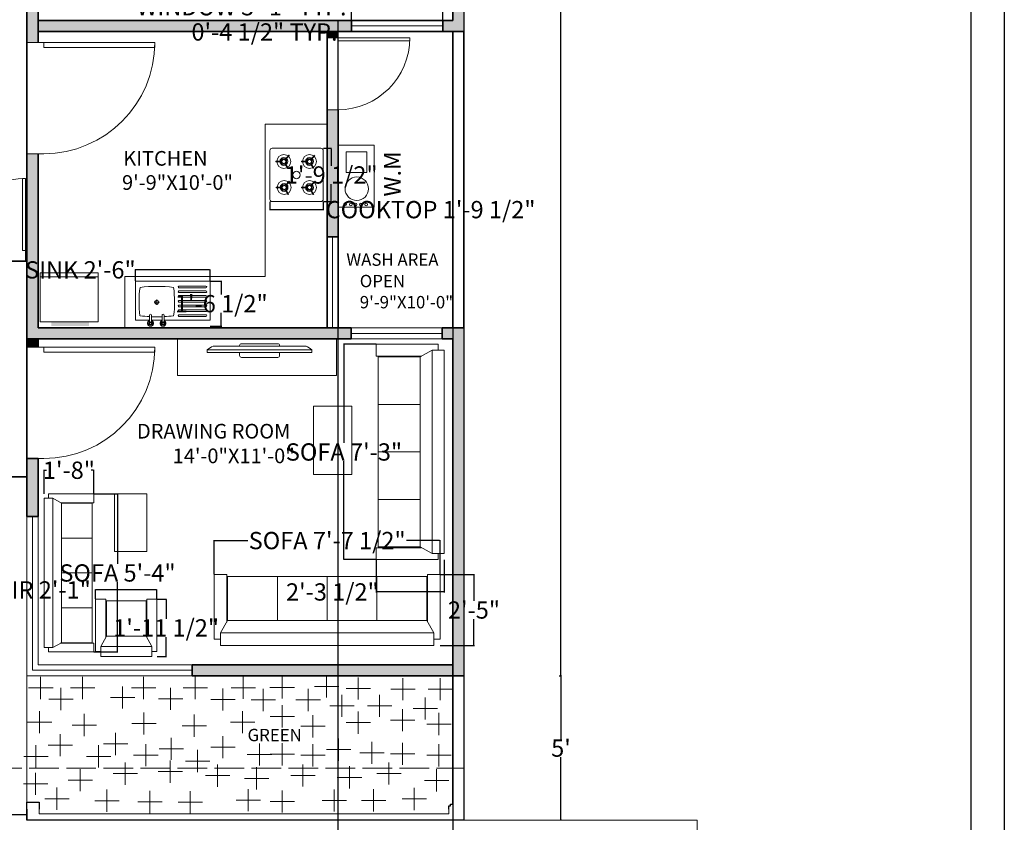
# Model space of a CAD drawing. Units: inches. Extents: x 0 to 4258, y 0 to 3769.
# Tile 18 of 30: x 3859 to 4258, y 2936 to 3261. Entities that reach past the tile are written whole.
import ezdxf

# ---------------------------------------------------------------- set-up
doc = ezdxf.new("R2010")
doc.units = ezdxf.units.IN
doc.header["$MEASUREMENT"] = 0
doc.linetypes.add('ACAD_ISO02W100', pattern=[15, 12, -3])
doc.layers.get('0').update_dxf_attribs({"color": 16})
for name, color, linetype, lineweight in [('A-ANNO-DIMS', 250, 'Continuous', 18), ('A-ANNO-TEXT', 250, 'Continuous', 18), ('A-ANNO-TTLB', 250, 'Continuous', 25), ('A-AREA-IDEN', 250, 'Continuous', 18), ('A-CASE', 150, 'Continuous', 18), ('A-EQPM', 8, 'Continuous', 18), ('A-FLOR-FIXT', 250, 'Continuous', 18), ('A-FLOR-OVHD', 150, 'ACAD_ISO02W100', 13), ('A-FLOR-STRS', 150, 'Continuous', 25), ('A-WALL-PATT', 16, 'Continuous', 13), ('C-PROP', 150, 'Continuous', 25), ('C-ROAD', 250, 'Continuous', 18), ('doors', 250, 'Continuous', 18), ('furniture', 13, 'Continuous', 18), ('L-PLNT-GRND', 102, 'Continuous', 13), ('walls', 251, 'Continuous', 35), ('windows', 121, 'Continuous', 18)]:
    doc.layers.add(name, color=color, linetype=linetype, lineweight=lineweight)
doc.styles.get("Standard").update_dxf_attribs({"font": 'arial.ttf'})
doc.dimstyles.get("Standard").update_dxf_attribs({"dimtxt": 7, "dimasz": 0.18, "dimexe": 0.18, "dimexo": 0.0625, "dimgap": 0.09, "dimtad": 0, "dimtih": 1, "dimtoh": 1, "dimzin": 0, "dimdsep": 46, "dimlunit": 3, "dimtxsty": 'Standard', "dimcen": 0.09, "dimadec": 0, "dimazin": 0, "dimtfac": 1, "dimtofl": 0, "dimtmove": 0, "dimatfit": 3, "dimfxl": 1, "dimtolj": 1, "dimtzin": 0, "dimarcsym": 0})

# ---------------------------------------------------------------- blocks, each defined once
blk = doc.blocks.new('FABRIC SOFA 4S')
at = {"layer": 'furniture'}
for p, q in [((3, 54), (34, 54)), ((3, 51), (3, 54)), ((34, 48), (34, 54)), ((0, -51), (0, 51)), ((6, 51), (0, 51)), ((6, -51), (6, 51)), ((12, 47.63), (6, 51)), ((11.14, 48), (34, 48)), ((33, 23.81), (12, 23.81)), ((33, 0), (12, 0)), ((33, -23.81), (12, -23.81)), ((6, -51), (0, -51)), ((3, -54), (3, -51)), ((6, -51), (12, -47.63)), ((11.54, -48), (34, -48)), ((34, -48), (34, -54)), ((3, -54), (34, -54))]:
    blk.add_line(p, q, dxfattribs=at)
blk.add_lwpolyline([(12, -47.63), (12, 47.63), (33, 47.63), (33, -47.63)], close=True, dxfattribs=at)
blk = doc.blocks.new('A$C799204C7')
for p, q in [((0, 34.2), (17.99, 34.2)), ((0, 0), (0, 34.2)), ((2.32, 20.01), (2.32, 32.27)), ((3.13, 20.01), (3.13, 32.27)), ((4.48, 20.01), (4.48, 32.27)), ((5.29, 20.01), (5.29, 32.27)), ((6.64, 20.01), (6.64, 32.27)), ((7.45, 20.01), (7.45, 32.27)), ((8.85, 20.01), (8.85, 32.27)), ((9.66, 20.01), (9.66, 32.27)), ((11.01, 20.01), (11.01, 32.27)), ((11.82, 20.01), (11.82, 32.27)), ((13.22, 20.01), (13.22, 32.27)), ((14.03, 20.01), (14.03, 32.27)), ((15.42, 20.01), (15.42, 32.27)), ((16.24, 20.01), (16.24, 32.27)), ((17.99, 13.08), (17.99, 34.2)), ((8.52, 9.77), (10.9, 9.77)), ((9.73, 11), (9.73, 8.54)), ((18.59, 13.08), (15.71, 13.08)), ((15.71, 12.17), (18.59, 12.17)), ((17.99, 7.36), (17.99, 12.17)), ((18.59, 7.36), (15.71, 7.36)), ((15.71, 6.45), (18.59, 6.45)), ((17.99, 0), (17.99, 6.45)), ((0, 0), (17.99, 0))]:
    blk.add_line(p, q)
for centre, radius in [((9.7, 9.77), 0.916), ((19.38, 12.62), 0.684), ((19.38, 12.62), 0.456), ((19.38, 6.91), 0.684), ((19.38, 6.91), 0.456)]:
    blk.add_circle(centre, radius)
for centre, radius, start, end in [((2.72, 32.27), 0.407, 0, 180), ((4.88, 32.27), 0.407, 0, 180), ((7.05, 32.27), 0.407, 0, 180), ((9.25, 32.27), 0.407, 0, 180), ((11.42, 32.27), 0.407, 0, 180), ((13.62, 32.27), 0.407, 0, 180), ((15.83, 32.27), 0.407, 0, 180), ((2.72, 20.01), 0.407, 180, 0), ((4.88, 20.01), 0.407, 180, 0), ((7.05, 20.01), 0.407, 180, 0), ((9.25, 20.01), 0.407, 180, 0), ((11.42, 20.01), 0.407, 180, 0), ((13.62, 20.01), 0.407, 180, 0), ((15.83, 20.01), 0.407, 180, 0), ((67.33, 9.77), 64.88, 173.1952, 186.8048), ((9.53, -30.19), 48.1, 82.3437, 97.8966), ((-48.51, 9.77), 64.88, 2.9208, 6.8048), ((19.38, 12.62), 1.37, 199.6514, 160.3603), ((15.71, 12.62), 0.456, 90, 270), ((-48.51, 9.77), 64.88, 357.8723, 2.115), ((19.38, 12.62), 0.911, 210.3431, 149.7554), ((15.71, 6.91), 0.456, 90, 270), ((-48.51, 9.77), 64.88, 353.1952, 357.0665), ((19.38, 6.91), 1.37, 199.6514, 160.3603), ((19.38, 6.91), 0.911, 210.3431, 149.7554), ((9.53, 49.73), 48.1, 262.1034, 277.6563)]:
    blk.add_arc(centre, radius, start, end)
blk = doc.blocks.new('sink')
at = {"layer": 'furniture'}
for p, q in [((8718164203.894819, -1433730582.369047), (8718164201.504578, -1433730582.369047)), ((8718164202.684322, -1433730581.131674), (8718164202.684322, -1433730583.598095)), ((8718164196.150837, -1433730592.638258), (8718164196.150837, -1433730604.938997)), ((8718164196.967728, -1433730592.638258), (8718164196.967728, -1433730604.938997)), ((8718164198.365185, -1433730592.638258), (8718164198.365185, -1433730604.938997)), ((8718164199.182076, -1433730592.638258), (8718164199.182076, -1433730604.938997)), ((8718164200.579533, -1433730592.638258), (8718164200.579533, -1433730604.938997)), ((8718164201.396423, -1433730592.638258), (8718164201.396423, -1433730604.938997)), ((8718164202.748692, -1433730592.638258), (8718164202.748692, -1433730604.938997)), ((8718164203.565582, -1433730592.638258), (8718164203.565582, -1433730604.938997)), ((8718164204.963041, -1433730592.638258), (8718164204.963041, -1433730604.938997)), ((8718164205.779934, -1433730592.638258), (8718164205.779934, -1433730604.938997)), ((8718164207.1322, -1433730592.638258), (8718164207.1322, -1433730604.938997)), ((8718164207.949093, -1433730592.638258), (8718164207.949093, -1433730604.938997)), ((8718164209.301359, -1433730592.638258), (8718164209.301359, -1433730604.938997)), ((8718164210.118252, -1433730592.638258), (8718164210.118252, -1433730604.938997))]:
    blk.add_line(p, q, dxfattribs=at)
for centre, radius in [((8718164192.998869, -1433730579.495552), 0.685789), ((8718164192.998869, -1433730579.495552), 0.457192), ((8718164192.998869, -1433730585.228166), 0.68579), ((8718164192.998869, -1433730585.228166), 0.68579), ((8718164192.998869, -1433730585.228166), 0.457192), ((8718164202.715019, -1433730582.369047), 0.919003)]:
    blk.add_circle(centre, radius, dxfattribs=at)
for centre, radius, start, end in [((8718164196.559284, -1433730592.638258), 0.41045, 354.3355999, 185.6644001), ((8718164198.77363, -1433730592.638258), 0.41045, 354.3355999, 185.6644001), ((8718164200.98798, -1433730592.638258), 0.41045, 354.3355999, 185.6644001), ((8718164203.157139, -1433730592.638258), 0.41045, 354.3355999, 185.6644001), ((8718164205.371487, -1433730592.638258), 0.41045, 354.3355999, 185.6644001), ((8718164207.540646, -1433730592.640262), 0.41045, 354.3355999, 185.6644001), ((8718164209.709805, -1433730592.640262), 0.41045, 354.3355999, 185.6644001), ((8718164196.559284, -1433730604.938997), 0.408445, 180, 0), ((8718164198.77363, -1433730604.938997), 0.408445, 180, 0), ((8718164200.98798, -1433730604.938997), 0.408445, 180, 0), ((8718164203.157139, -1433730604.938997), 0.408445, 180, 0), ((8718164205.371487, -1433730604.938997), 0.408445, 180, 0), ((8718164207.540646, -1433730604.938997), 0.408445, 180, 0), ((8718164209.709805, -1433730604.938997), 0.408445, 180, 0)]:
    blk.add_arc(centre, radius, start, end, dxfattribs=at)
at = {"layer": 'furniture', "xscale": 1.0032, "yscale": 1.0032, "zscale": 1.0032, "rotation": 180}
blk.add_blockref('A$C799204C7', (8718164212.441259, -1433730572.566334), dxfattribs=at)
blk = doc.blocks.new('washbasin')
at = {"layer": 'furniture'}
blk.add_blockref('sink', (-8718164214.119328, 1433730589.721069), dxfattribs=at)
blk = doc.blocks.new('4bstove')
at = {"layer": 'furniture'}
for p, q in [((1452.73, 1446.21), (1452.73, 1448.61)), ((1452.98, 1446.22), (1452.98, 1448.61)), ((1464.44, 1446.34), (1464.44, 1448.73)), ((1464.69, 1446.34), (1464.69, 1448.73)), ((1451.74, 1444.45), (1449.67, 1443.25)), ((1451.87, 1444.23), (1449.79, 1443.04)), ((1453.75, 1444.08), (1455.58, 1442.54)), ((1453.91, 1444.27), (1455.74, 1442.73)), ((1463.45, 1444.58), (1461.38, 1443.38)), ((1463.57, 1444.36), (1461.5, 1443.17)), ((1465.46, 1444.21), (1467.29, 1442.67)), ((1465.62, 1444.4), (1467.45, 1442.86)), ((1452.69, 1434.81), (1452.69, 1437.2)), ((1452.94, 1434.81), (1452.94, 1437.2)), ((1464.44, 1434.81), (1464.44, 1437.2)), ((1464.69, 1434.81), (1464.69, 1437.2)), ((1451.7, 1433.04), (1449.63, 1431.85)), ((1451.82, 1432.83), (1449.75, 1431.63)), ((1453.71, 1432.67), (1455.54, 1431.13)), ((1453.87, 1432.86), (1455.7, 1431.33)), ((1463.45, 1433.04), (1461.38, 1431.85)), ((1463.57, 1432.83), (1461.5, 1431.63)), ((1465.46, 1432.67), (1467.29, 1431.13)), ((1465.62, 1432.86), (1467.45, 1431.33))]:
    blk.add_line(p, q, dxfattribs=at)
for points in [[(1447.5, 1427.38), (1469.5, 1427.38, 0.414214), (1470.5, 1428.38), (1470.5, 1450.38, 0.414214), (1469.5, 1451.38), (1447.5, 1451.38, 0.414214), (1446.5, 1450.38), (1446.5, 1428.38, 0.414214)], [(1453.75, 1444.97, 1), (1452, 1444.97, 1)], [(1465.46, 1445.1, 1), (1463.71, 1445.1, 1)], [(1453.71, 1433.56, 1), (1451.96, 1433.56, 1)], [(1465.46, 1433.56, 1), (1463.71, 1433.56, 1)]]:
    blk.add_lwpolyline(points, format="xyb", close=True, dxfattribs=at)
for points in [[(1454.12, 1444.97, 1), (1451.62, 1444.97, 1), (1454.12, 1444.97, 1)], [(1465.83, 1445.1, 1), (1463.33, 1445.1, 1), (1465.83, 1445.1, 1)], [(1454.08, 1433.56, 1), (1451.58, 1433.56, 1), (1454.08, 1433.56, 1)], [(1465.83, 1433.56, 1), (1463.33, 1433.56, 1), (1465.83, 1433.56, 1)]]:
    blk.add_lwpolyline(points, format="xyb", dxfattribs=at)
for centre, radius in [((1452.87, 1444.97), 3.14), ((1452.87, 1444.97), 1.75), ((1464.58, 1445.1), 3.14), ((1464.58, 1445.1), 1.75), ((1458.5, 1439.38), 1.67), ((1452.83, 1433.56), 3.14), ((1464.58, 1433.56), 3.14), ((1452.83, 1433.56), 1.75), ((1464.58, 1433.56), 1.75)]:
    blk.add_circle(centre, radius, dxfattribs=at)
for centre, start, end in [((1452.87, 1444.97), 88.2645, 92.2039), ((1464.58, 1445.1), 88.2645, 92.2039), ((1452.87, 1444.97), 208.188, 212.1274), ((1452.87, 1444.97), 318.1018, 322.0412), ((1464.58, 1445.1), 208.188, 212.1274), ((1464.58, 1445.1), 318.1018, 322.0412), ((1452.83, 1433.56), 88.2645, 92.2039), ((1464.58, 1433.56), 88.2645, 92.2039)]:
    blk.add_arc(centre, 3.64, start, end, dxfattribs=at)
blk = doc.blocks.new('stove')
at = {"layer": 'furniture', "xscale": 0.9, "yscale": 0.9, "zscale": 0.9, "rotation": 89.99999999999999}
blk.add_blockref('4bstove', (1295.44, -1312.65), dxfattribs=at)
blk = doc.blocks.new('FABRIC SOFA 1S')
at = {"layer": 'furniture'}
for p, q in [((3, 18.12), (34, 18.12)), ((3, 15.12), (3, 18.12)), ((34, 12.12), (34, 18.12)), ((0, -15.12), (0, 15.12)), ((6, 15.12), (0, 15.12)), ((6, -15.12), (6, 15.12)), ((12, 11.75), (6, 15.12)), ((11.33, 12.12), (34, 12.12)), ((6, -15.12), (0, -15.12)), ((3, -18.12), (3, -15.12)), ((6, -15.12), (12, -11.75)), ((11.33, -12.12), (34, -12.12)), ((34, -12.12), (34, -18.12)), ((3, -18.12), (34, -18.12))]:
    blk.add_line(p, q, dxfattribs=at)
blk.add_lwpolyline([(12, -11.75), (12, 11.75), (33, 11.75), (33, -11.75)], close=True, dxfattribs=at)
blk = doc.blocks.new('PLASMA-LARGE')
at = {"layer": 'furniture'}
for p, q in [((-7.26, 0), (7.26, 0)), ((-21, -2.5), (21, -2.5)), ((-21, -2.5), (-21, -3.5)), ((-21, -3.5), (21, -3.5)), ((-18.61, -1), (18.61, -1)), ((-8, -1), (-8, -0.74)), ((-8, -3.5), (-8, -4.76)), ((8, -1), (8, -0.74)), ((8, -3.5), (8, -4.76)), ((21, -2.5), (21, -3.5)), ((-7.26, -5.5), (7.26, -5.5))]:
    blk.add_line(p, q, dxfattribs=at)
for centre, radius, start, end in [((-7.26, -0.74), 0.744, 90, 180), ((7.26, -0.74), 0.744, 0, 90), ((-13.97, -11.05), 11.07, 114.7602, 129.4175), ((13.97, -11.05), 11.07, 50.5825, 65.2398), ((-7.26, -4.76), 0.744, 180, 270), ((7.26, -4.76), 0.744, 270, 0)]:
    blk.add_arc(centre, radius, start, end, dxfattribs=at)
blk = doc.blocks.new('*U23')
for p, q in [((0, 0), (0, -6)), ((40, 0), (40, -6))]:
    blk.add_line(p, q)
blk.add_lwpolyline([(0, 0), (0, 40), (1.75, 40), (1.75, 0)], close=True)
blk.add_arc((0, 0), 40, 0, 90)
blk = doc.blocks.new('*D26')
at = {"layer": 'A-ANNO-DIMS', "color": 0, "lineweight": -2, "transparency": 16777216}
for p, q in [((4077.41, 3656.79), (4078.27, 3656.79)), ((4078.09, 3656.61), (4078.09, 3329.69)), ((4078.09, 2995.47), (4078.09, 3322.39)), ((4077.41, 2995.29), (4078.27, 2995.29))]:
    blk.add_line(p, q, dxfattribs=at)
at = {"layer": 'A-ANNO-DIMS', "color": 0, "transparency": 16777216}
for points in [[(4078.06, 3656.61), (4078.12, 3656.61), (4078.09, 3656.79)], [(4078.06, 2995.47), (4078.12, 2995.47), (4078.09, 2995.29)]]:
    blk.add_solid(points, dxfattribs=at)
at = {"layer": 'Defpoints', "color": 0, "transparency": 16777216}
for p in [(4077.35, 3656.79), (4077.35, 2995.29), (4078.09, 2995.29)]:
    blk.add_point(p, dxfattribs=at)
at = {"layer": 'A-ANNO-DIMS', "color": 0, "transparency": 16777216, "insert": (4078.09, 3326.04), "char_height": 7, "attachment_point": 5}
blk.add_mtext("\\A1;55'", dxfattribs=at)
blk = doc.blocks.new('*D27')
at = {"layer": 'A-ANNO-DIMS', "color": 0, "lineweight": -2, "transparency": 16777216}
for p, q in [((4078.25, 2995.29), (4077.91, 2995.29)), ((4078.09, 2995.11), (4078.09, 2969.69)), ((4078.09, 2936.97), (4078.09, 2962.39)), ((4078.25, 2936.79), (4077.91, 2936.79))]:
    blk.add_line(p, q, dxfattribs=at)
at = {"layer": 'A-ANNO-DIMS', "color": 0, "transparency": 16777216}
for points in [[(4078.06, 2995.11), (4078.12, 2995.11), (4078.09, 2995.29)], [(4078.06, 2936.97), (4078.12, 2936.97), (4078.09, 2936.79)]]:
    blk.add_solid(points, dxfattribs=at)
at = {"layer": 'Defpoints', "color": 0, "transparency": 16777216}
for p in [(4078.31, 2995.29), (4078.09, 2936.79), (4078.31, 2936.79)]:
    blk.add_point(p, dxfattribs=at)
at = {"layer": 'A-ANNO-DIMS', "color": 0, "transparency": 16777216, "insert": (4078.09, 2966.04), "char_height": 7, "width": 37.9222, "attachment_point": 5}
blk.add_mtext("\\A1;5'", dxfattribs=at)
blk = doc.blocks.new('WINDOW-37IN')
for p, q in [((0, 4.5), (36.9, 4.5)), ((0, 2.25), (36.9, 2.25)), ((0, 0), (36.9, 0))]:
    blk.add_line(p, q)
blk = doc.blocks.new('TV-CONSOLE-CABINET')
for p, q in [((0, 0), (0, 64.44)), ((0, 64.44), (14.9, 64.44)), ((14.9, 0), (0, 0))]:
    blk.add_line(p, q)
blk = doc.blocks.new('LAWN-COVER-MARK')
for p, q in [((4.88, 8.97), (4.88, 0)), ((0, 4.49), (9.88, 4.49))]:
    blk.add_line(p, q)
blk = doc.blocks.new('*D40')
at = {"layer": 'A-ANNO-DIMS', "color": 0, "lineweight": -2, "transparency": 16777216}
for p, q in [((3937.65, 3036.44), (3937.65, 3050.28)), ((3937.83, 3050.1), (3951.19, 3050.1)), ((4028.95, 3050.1), (4015.59, 3050.1)), ((4029.13, 3036.44), (4029.13, 3050.28))]:
    blk.add_line(p, q, dxfattribs=at)
at = {"layer": 'A-ANNO-DIMS', "color": 0, "transparency": 16777216}
for points in [[(3937.83, 3050.13), (3937.83, 3050.07), (3937.65, 3050.1)], [(4028.95, 3050.13), (4028.95, 3050.07), (4029.13, 3050.1)]]:
    blk.add_solid(points, dxfattribs=at)
at = {"layer": 'Defpoints', "color": 0, "transparency": 16777216}
for p in [(3937.65, 3050.1), (3937.65, 3036.38), (4029.13, 3036.38)]:
    blk.add_point(p, dxfattribs=at)
at = {"layer": 'A-ANNO-DIMS', "color": 0, "transparency": 16777216, "insert": (3983.39, 3050.1), "char_height": 7, "attachment_point": 5}
blk.add_mtext('\\A1;SOFA 7\'-7 1/2"', dxfattribs=at)
blk = doc.blocks.new('*D41')
at = {"layer": 'A-ANNO-DIMS', "color": 0, "lineweight": -2, "transparency": 16777216}
for p, q in [((4029.19, 3036.38), (4043.03, 3036.38)), ((4042.85, 3036.2), (4042.85, 3025.65)), ((4042.85, 3007.76), (4042.85, 3018.32)), ((4029.19, 3007.58), (4043.03, 3007.58))]:
    blk.add_line(p, q, dxfattribs=at)
at = {"layer": 'A-ANNO-DIMS', "color": 0, "transparency": 16777216}
for points in [[(4042.82, 3036.2), (4042.88, 3036.2), (4042.85, 3036.38)], [(4042.82, 3007.76), (4042.88, 3007.76), (4042.85, 3007.58)]]:
    blk.add_solid(points, dxfattribs=at)
at = {"layer": 'Defpoints', "color": 0, "transparency": 16777216}
for p in [(4029.13, 3036.38), (4042.85, 3036.38), (4029.13, 3007.58)]:
    blk.add_point(p, dxfattribs=at)
at = {"layer": 'A-ANNO-DIMS', "color": 0, "transparency": 16777216, "insert": (4042.85, 3021.98), "char_height": 7, "attachment_point": 5}
blk.add_mtext('\\A1;2\'-5"', dxfattribs=at)
blk = doc.blocks.new('*D42')
at = {"layer": 'A-ANNO-DIMS', "color": 0, "lineweight": -2, "transparency": 16777216}
for p, q in [((4003.23, 3129.61), (3990.02, 3129.61)), ((3990.2, 3129.43), (3990.2, 3089.71)), ((3990.2, 3042.56), (3990.2, 3082.28)), ((4003.23, 3042.38), (3990.02, 3042.38))]:
    blk.add_line(p, q, dxfattribs=at)
at = {"layer": 'A-ANNO-DIMS', "color": 0, "transparency": 16777216}
for points in [[(3990.17, 3129.43), (3990.23, 3129.43), (3990.2, 3129.61)], [(3990.17, 3042.56), (3990.23, 3042.56), (3990.2, 3042.38)]]:
    blk.add_solid(points, dxfattribs=at)
at = {"layer": 'Defpoints', "color": 0, "transparency": 16777216}
for p in [(3990.2, 3129.61), (4003.29, 3129.61), (4003.29, 3042.38)]:
    blk.add_point(p, dxfattribs=at)
at = {"layer": 'A-ANNO-DIMS', "color": 0, "transparency": 16777216, "insert": (3990.2, 3085.99), "char_height": 7, "attachment_point": 5}
blk.add_mtext('\\A1;SOFA 7\'-3"', dxfattribs=at)
blk = doc.blocks.new('*D43')
at = {"layer": 'A-ANNO-DIMS', "color": 0, "lineweight": -2, "transparency": 16777216}
for p, q in [((4003.29, 3042.32), (4003.29, 3029.11)), ((4030.75, 3042.32), (4030.75, 3029.11)), ((4003.29, 3029.29), (4003.11, 3029.29)), ((4030.57, 3029.29), (4003.47, 3029.29))]:
    blk.add_line(p, q, dxfattribs=at)
at = {"layer": 'A-ANNO-DIMS', "color": 0, "transparency": 16777216}
for points in [[(4003.47, 3029.32), (4003.47, 3029.26), (4003.29, 3029.29)], [(4030.57, 3029.32), (4030.57, 3029.26), (4030.75, 3029.29)]]:
    blk.add_solid(points, dxfattribs=at)
at = {"layer": 'Defpoints', "color": 0, "transparency": 16777216}
for p in [(4003.29, 3042.38), (4030.75, 3042.38), (4003.29, 3029.29)]:
    blk.add_point(p, dxfattribs=at)
at = {"layer": 'A-ANNO-DIMS', "color": 0, "transparency": 16777216, "insert": (3985.5, 3029.29), "char_height": 7, "attachment_point": 5}
blk.add_mtext('\\A1;2\'-3 1/2"', dxfattribs=at)
blk = doc.blocks.new('*D44')
at = {"layer": 'A-ANNO-DIMS', "color": 0, "lineweight": -2, "transparency": 16777216}
for p, q in [((3888.92, 3068.99), (3898.64, 3068.99)), ((3898.46, 3068.81), (3898.46, 3040.69)), ((3898.46, 3005.15), (3898.46, 3033.27)), ((3888.92, 3004.97), (3898.64, 3004.97))]:
    blk.add_line(p, q, dxfattribs=at)
at = {"layer": 'A-ANNO-DIMS', "color": 0, "transparency": 16777216}
for points in [[(3898.43, 3068.81), (3898.49, 3068.81), (3898.46, 3068.99)], [(3898.43, 3005.15), (3898.49, 3005.15), (3898.46, 3004.97)]]:
    blk.add_solid(points, dxfattribs=at)
at = {"layer": 'Defpoints', "color": 0, "transparency": 16777216}
for p in [(3888.85, 3068.99), (3888.85, 3004.97), (3898.46, 3004.97)]:
    blk.add_point(p, dxfattribs=at)
at = {"layer": 'A-ANNO-DIMS', "color": 0, "transparency": 16777216, "insert": (3898.46, 3036.98), "char_height": 7, "attachment_point": 5}
blk.add_mtext('\\A1;SOFA 5\'-4"', dxfattribs=at)
blk = doc.blocks.new('*D45')
at = {"layer": 'A-ANNO-DIMS', "color": 0, "lineweight": -2, "transparency": 16777216}
for p, q in [((3868.7, 3069.05), (3868.7, 3078.77)), ((3868.88, 3078.59), (3869.71, 3078.59)), ((3888.67, 3078.59), (3887.84, 3078.59)), ((3888.85, 3069.05), (3888.85, 3078.77))]:
    blk.add_line(p, q, dxfattribs=at)
at = {"layer": 'A-ANNO-DIMS', "color": 0, "transparency": 16777216}
for points in [[(3868.88, 3078.62), (3868.88, 3078.56), (3868.7, 3078.59)], [(3888.67, 3078.62), (3888.67, 3078.56), (3888.85, 3078.59)]]:
    blk.add_solid(points, dxfattribs=at)
at = {"layer": 'Defpoints', "color": 0, "transparency": 16777216}
for p in [(3888.85, 3078.59), (3868.7, 3068.99), (3888.85, 3068.99)]:
    blk.add_point(p, dxfattribs=at)
at = {"layer": 'A-ANNO-DIMS', "color": 0, "transparency": 16777216, "insert": (3878.78, 3078.59), "char_height": 7, "attachment_point": 5}
blk.add_mtext('\\A1;1\'-8"', dxfattribs=at)
blk = doc.blocks.new('*D52')
at = {"layer": 'A-ANNO-DIMS', "color": 0, "lineweight": -2, "transparency": 16777216}
for p, q in [((3889.6, 3030.12), (3889.42, 3030.12)), ((3889.6, 3026.46), (3889.6, 3030.3)), ((3914.27, 3030.12), (3889.78, 3030.12)), ((3914.45, 3026.46), (3914.45, 3030.3))]:
    blk.add_line(p, q, dxfattribs=at)
at = {"layer": 'A-ANNO-DIMS', "color": 0, "transparency": 16777216}
for points in [[(3889.78, 3030.15), (3889.78, 3030.09), (3889.6, 3030.12)], [(3914.27, 3030.15), (3914.27, 3030.09), (3914.45, 3030.12)]]:
    blk.add_solid(points, dxfattribs=at)
at = {"layer": 'Defpoints', "color": 0, "transparency": 16777216}
for p in [(3889.6, 3030.12), (3889.6, 3026.4), (3914.45, 3026.4)]:
    blk.add_point(p, dxfattribs=at)
at = {"layer": 'A-ANNO-DIMS', "color": 0, "transparency": 16777216, "insert": (3852.38, 3030.12), "char_height": 7, "attachment_point": 5}
blk.add_mtext('\\A1;ARMCHAIR 2\'-1"', dxfattribs=at)
blk = doc.blocks.new('*D53')
at = {"layer": 'A-ANNO-DIMS', "color": 0, "lineweight": -2, "transparency": 16777216}
for p, q in [((3914.51, 3026.4), (3918.35, 3026.4)), ((3918.17, 3026.22), (3918.17, 3018.45)), ((3918.17, 3003.27), (3918.17, 3011.03)), ((3914.51, 3003.09), (3918.35, 3003.09))]:
    blk.add_line(p, q, dxfattribs=at)
at = {"layer": 'A-ANNO-DIMS', "color": 0, "transparency": 16777216}
for points in [[(3918.14, 3026.22), (3918.2, 3026.22), (3918.17, 3026.4)], [(3918.14, 3003.27), (3918.2, 3003.27), (3918.17, 3003.09)]]:
    blk.add_solid(points, dxfattribs=at)
at = {"layer": 'Defpoints', "color": 0, "transparency": 16777216}
for p in [(3914.45, 3026.4), (3918.17, 3026.4), (3914.45, 3003.09)]:
    blk.add_point(p, dxfattribs=at)
at = {"layer": 'A-ANNO-DIMS', "color": 0, "transparency": 16777216, "insert": (3918.17, 3014.74), "char_height": 7, "attachment_point": 5}
blk.add_mtext('\\A1;1\'-11 1/2"', dxfattribs=at)
blk = doc.blocks.new('*D58')
at = {"layer": 'A-ANNO-DIMS', "color": 0, "lineweight": -2, "transparency": 16777216}
for p, q in [((3993.31, 3260.86), (3993.31, 3266.51)), ((4030.21, 3260.86), (4030.21, 3266.51)), ((3993.31, 3266.33), (3993.13, 3266.33)), ((4030.03, 3266.33), (3993.49, 3266.33))]:
    blk.add_line(p, q, dxfattribs=at)
at = {"layer": 'A-ANNO-DIMS', "color": 0, "transparency": 16777216}
for points in [[(3993.49, 3266.36), (3993.49, 3266.3), (3993.31, 3266.33)], [(4030.03, 3266.36), (4030.03, 3266.3), (4030.21, 3266.33)]]:
    blk.add_solid(points, dxfattribs=at)
at = {"layer": 'Defpoints', "color": 0, "transparency": 16777216}
for p in [(3993.31, 3266.33), (3993.31, 3260.79), (4030.21, 3260.79)]:
    blk.add_point(p, dxfattribs=at)
at = {"layer": 'A-ANNO-DIMS', "color": 0, "transparency": 16777216, "insert": (3948.75, 3266.33), "char_height": 7, "attachment_point": 5}
blk.add_mtext('\\A1;WINDOW 3\'-1" TYP.', dxfattribs=at)
blk = doc.blocks.new('*D59')
at = {"layer": 'A-ANNO-DIMS', "color": 0, "lineweight": -2, "transparency": 16777216}
for p, q in [((3993.24, 3260.79), (3987.59, 3260.79)), ((3987.77, 3260.61), (3987.77, 3256.47)), ((3993.24, 3256.29), (3987.59, 3256.29)), ((3987.77, 3256.11), (3987.59, 3256.11)), ((3987.77, 3256.29), (3987.77, 3256.11))]:
    blk.add_line(p, q, dxfattribs=at)
at = {"layer": 'A-ANNO-DIMS', "color": 0, "transparency": 16777216}
for points in [[(3987.74, 3260.61), (3987.8, 3260.61), (3987.77, 3260.79)], [(3987.74, 3256.47), (3987.8, 3256.47), (3987.77, 3256.29)]]:
    blk.add_solid(points, dxfattribs=at)
at = {"layer": 'Defpoints', "color": 0, "transparency": 16777216}
for p in [(3993.31, 3260.79), (3987.77, 3256.29), (3993.31, 3256.29)]:
    blk.add_point(p, dxfattribs=at)
at = {"layer": 'A-ANNO-DIMS', "color": 0, "transparency": 16777216, "insert": (3958.01, 3256.11), "char_height": 7, "attachment_point": 5}
blk.add_mtext('\\A1;0\'-4 1/2" TYP.', dxfattribs=at)
blk = doc.blocks.new('*D68')
at = {"layer": 'A-ANNO-DIMS', "color": 0, "lineweight": -2, "transparency": 16777216}
for p, q in [((3905.75, 3159.75), (3905.57, 3159.75)), ((3905.75, 3155.28), (3905.75, 3159.93)), ((3935.79, 3159.75), (3905.93, 3159.75)), ((3935.97, 3155.28), (3935.97, 3159.93))]:
    blk.add_line(p, q, dxfattribs=at)
at = {"layer": 'A-ANNO-DIMS', "color": 0, "transparency": 16777216}
for points in [[(3905.93, 3159.78), (3905.93, 3159.72), (3905.75, 3159.75)], [(3935.79, 3159.78), (3935.79, 3159.72), (3935.97, 3159.75)]]:
    blk.add_solid(points, dxfattribs=at)
at = {"layer": 'Defpoints', "color": 0, "transparency": 16777216}
for p in [(3905.75, 3159.75), (3905.75, 3155.22), (3935.97, 3155.22)]:
    blk.add_point(p, dxfattribs=at)
at = {"layer": 'A-ANNO-DIMS', "color": 0, "transparency": 16777216, "insert": (3883.43, 3159.75), "char_height": 7, "attachment_point": 5}
blk.add_mtext('\\A1;SINK 2\'-6"', dxfattribs=at)
blk = doc.blocks.new('*D69')
at = {"layer": 'A-ANNO-DIMS', "color": 0, "lineweight": -2, "transparency": 16777216}
for p, q in [((3936.03, 3155.22), (3940.69, 3155.22)), ((3940.51, 3155.04), (3940.51, 3149.76)), ((3940.51, 3137.07), (3940.51, 3142.34)), ((3936.03, 3136.89), (3940.69, 3136.89))]:
    blk.add_line(p, q, dxfattribs=at)
at = {"layer": 'A-ANNO-DIMS', "color": 0, "transparency": 16777216}
for points in [[(3940.48, 3155.04), (3940.54, 3155.04), (3940.51, 3155.22)], [(3940.48, 3137.07), (3940.54, 3137.07), (3940.51, 3136.89)]]:
    blk.add_solid(points, dxfattribs=at)
at = {"layer": 'Defpoints', "color": 0, "transparency": 16777216}
for p in [(3935.97, 3155.22), (3940.51, 3155.22), (3935.97, 3136.89)]:
    blk.add_point(p, dxfattribs=at)
at = {"layer": 'A-ANNO-DIMS', "color": 0, "transparency": 16777216, "insert": (3940.51, 3146.05), "char_height": 7, "attachment_point": 5}
blk.add_mtext('\\A1;1\'-6 1/2"', dxfattribs=at)
blk = doc.blocks.new('*D70')
at = {"layer": 'A-ANNO-DIMS', "color": 0, "lineweight": -2, "transparency": 16777216}
for p, q in [((3960.18, 3187.33), (3960.18, 3183.97)), ((3981.78, 3187.33), (3981.78, 3183.97)), ((3960.36, 3184.15), (3981.6, 3184.15)), ((3981.78, 3184.15), (3981.96, 3184.15))]:
    blk.add_line(p, q, dxfattribs=at)
at = {"layer": 'A-ANNO-DIMS', "color": 0, "transparency": 16777216}
for points in [[(3960.36, 3184.18), (3960.36, 3184.12), (3960.18, 3184.15)], [(3981.6, 3184.18), (3981.6, 3184.12), (3981.78, 3184.15)]]:
    blk.add_solid(points, dxfattribs=at)
at = {"layer": 'Defpoints', "color": 0, "transparency": 16777216}
for p in [(3960.18, 3187.39), (3981.78, 3187.39), (3981.78, 3184.15)]:
    blk.add_point(p, dxfattribs=at)
at = {"layer": 'A-ANNO-DIMS', "color": 0, "transparency": 16777216, "insert": (4025.28, 3184.15), "char_height": 7, "attachment_point": 5}
blk.add_mtext('\\A1;COOKTOP 1\'-9 1/2"', dxfattribs=at)
blk = doc.blocks.new('*D71')
at = {"layer": 'A-ANNO-DIMS', "color": 0, "lineweight": -2, "transparency": 16777216}
for p, q in [((3981.85, 3208.99), (3985.2, 3208.99)), ((3985.02, 3208.81), (3985.02, 3201.9)), ((3985.02, 3187.57), (3985.02, 3194.48)), ((3981.85, 3187.39), (3985.2, 3187.39))]:
    blk.add_line(p, q, dxfattribs=at)
at = {"layer": 'A-ANNO-DIMS', "color": 0, "transparency": 16777216}
for points in [[(3984.99, 3208.81), (3985.05, 3208.81), (3985.02, 3208.99)], [(3984.99, 3187.57), (3985.05, 3187.57), (3985.02, 3187.39)]]:
    blk.add_solid(points, dxfattribs=at)
at = {"layer": 'Defpoints', "color": 0, "transparency": 16777216}
for p in [(3981.78, 3208.99), (3985.02, 3208.99), (3981.78, 3187.39)]:
    blk.add_point(p, dxfattribs=at)
at = {"layer": 'A-ANNO-DIMS', "color": 0, "transparency": 16777216, "insert": (3985.02, 3198.19), "char_height": 7, "attachment_point": 5}
blk.add_mtext('\\A1;1\'-9 1/2"', dxfattribs=at)
blk = doc.blocks.new('*D72')
at = {"layer": 'A-ANNO-DIMS', "color": 0, "lineweight": -2, "transparency": 16777216}
for p, q in [((4034.3, 3256.23), (4034.3, 2818.78)), ((3987.71, 3253.71), (3987.71, 2818.78)), ((3987.89, 2818.96), (3990.74, 2818.96)), ((4034.12, 2818.96), (4031.27, 2818.96))]:
    blk.add_line(p, q, dxfattribs=at)
at = {"layer": 'A-ANNO-DIMS', "color": 0, "transparency": 16777216}
for points in [[(3987.89, 2818.99), (3987.89, 2818.93), (3987.71, 2818.96)], [(4034.12, 2818.99), (4034.12, 2818.93), (4034.3, 2818.96)]]:
    blk.add_solid(points, dxfattribs=at)
at = {"layer": 'Defpoints', "color": 0, "transparency": 16777216}
for p in [(4034.3, 3256.29), (3987.71, 3253.78), (4034.3, 2818.96)]:
    blk.add_point(p, dxfattribs=at)
at = {"layer": 'A-ANNO-DIMS', "color": 0, "transparency": 16777216, "insert": (4011.01, 2818.96), "char_height": 7, "attachment_point": 5}
blk.add_mtext('\\A1;3\'-10 1/2"', dxfattribs=at)

msp = doc.modelspace()

# ---------------------------------------------------------------- hatches: boundary and pattern name
at = {"layer": 'A-EQPM'}
h = msp.add_hatch(color=256, dxfattribs=at)
h.dxf.hatch_style = 1
h.paths.add_polyline_path([(3886.878, 3137.07), (3886.878, 3138.634), (3871.646, 3138.634), (3871.646, 3137.07)])
at = {"layer": 'A-WALL-PATT'}
h = msp.add_hatch(color=256, dxfattribs=at)
h.dxf.hatch_style = 1
h.paths.add_polyline_path([(3866.304, 3343.984), (3861.804, 3343.984), (3861.804, 3251.848), (3866.304, 3251.848)])
h.paths.add_polyline_path([(3881.946, 3330.642), (3866.304, 3330.642), (3866.304, 3326.142), (3881.946, 3326.142)])
h.paths.add_polyline_path([(4038.804, 3656.793), (3933.804, 3656.793), (3933.804, 3638.769), (3938.304, 3638.769), (3938.304, 3652.293), (4034.304, 3652.293), (4034.304, 3260.793), (4030.207, 3260.793), (4030.207, 3256.293), (4038.804, 3256.293)])
h = msp.add_hatch(color=256, dxfattribs=at)
h.dxf.hatch_style = 1
h.paths.add_polyline_path([(3993.305, 3260.793), (3866.304, 3260.793), (3866.304, 3256.293), (3993.305, 3256.293)])
h.paths.add_polyline_path([(4038.804, 3136.293), (4030.04, 3136.293), (4030.04, 3131.793), (4034.304, 3131.793), (4034.304, 2995.293), (4038.804, 2995.293)])
h.paths.add_polyline_path([(4034.304, 2999.793), (3928.723, 2999.793), (3928.723, 2995.293), (4034.304, 2995.293)])
h.paths.add_polyline_path([(4014.899, 3187.712), (4014.899, 3210.714), (4004.662, 3210.714), (4004.662, 3187.712)], flags=9)
h = msp.add_hatch(color=256, dxfattribs=at)
h.dxf.hatch_style = 1
h.paths.add_polyline_path([(3987.712, 3256.293), (3983.335, 3256.293), (3983.335, 3253.777), (3987.712, 3253.777)])
h = msp.add_hatch(color=256, dxfattribs=at)
h.dxf.hatch_style = 1
h.paths.add_polyline_path([(3866.304, 3206.808), (3861.804, 3206.808), (3861.804, 3163.293), (3861.804, 3131.793), (3993.138, 3131.793), (3993.138, 3136.293), (3866.304, 3136.293)])
h.paths.add_polyline_path([(3866.304, 3083.341), (3861.804, 3083.341), (3861.804, 3059.818), (3866.304, 3059.818)])
edge = h.paths.add_edge_path()
edge.add_line((3987.712, 3224.597), (3983.335, 3224.597))
edge.add_line((3983.335, 3224.597), (3983.335, 3173.195))
edge.add_line((3983.335, 3173.195), (3987.835, 3173.195))
edge.add_line((3987.835, 3173.195), (3987.835, 3224.597))
edge.add_arc((3987.712, 3253.777), 29.18, 270, 270.24143, ccw=False)
h = msp.add_hatch(color=256, dxfattribs=at)
h.dxf.hatch_style = 1
h.paths.add_polyline_path([(3866.304, 3131.793), (3861.804, 3131.793), (3861.804, 3128.38), (3866.304, 3128.38)])

# ---------------------------------------------------------------- linework, layer by layer
at = {"layer": 'A-ANNO-TTLB'}
for p, q in [((4257.673, 3768.679), (4257.673, 2749.714)), ((4244.279, 2762.335), (4244.279, 3758.41))]:
    msp.add_line(p, q, dxfattribs=at)
at = {"layer": 'A-CASE'}
for p, q in [((3958.264, 3157.012), (3958.264, 3218.827)), ((3958.264, 3218.827), (3983.335, 3218.827)), ((3901.437, 3136.293), (3901.437, 3157.012)), ((3901.437, 3157.012), (3958.264, 3157.012))]:
    msp.add_line(p, q, dxfattribs=at)
at = {"layer": 'A-EQPM'}
for p, q in [((4002.436, 3210.2), (3987.835, 3210.2)), ((3991.119, 3199.188), (3991.119, 3207.524)), ((3991.119, 3207.524), (3999.462, 3207.524)), ((3999.462, 3207.524), (3999.462, 3199.188)), ((4002.436, 3185.144), (4002.436, 3210.2)), ((3999.462, 3199.188), (3991.119, 3199.188)), ((4002.436, 3185.144), (3987.835, 3185.144)), ((3987.835, 3179.127), (3987.835, 3179.127)), ((3867.157, 3158.559), (3890.621, 3158.559)), ((3867.157, 3138.634), (3867.157, 3158.559)), ((3867.157, 3156.965), (3890.621, 3156.965)), ((3890.621, 3158.559), (3890.621, 3138.634)), ((3890.621, 3138.634), (3867.157, 3138.634))]:
    msp.add_line(p, q, dxfattribs=at)
for centre, radius in [((3995.369, 3192.615), 4.752), ((3990.673, 3186.375), 0.542), ((3992.981, 3186.228), 0.542), ((3994.882, 3186.228), 0.542), ((3997.082, 3186.228), 0.542), ((3999.174, 3186.228), 0.542)]:
    msp.add_circle(centre, radius, dxfattribs=at)
at = {"layer": 'A-FLOR-OVHD'}
msp.add_line((3832.744, 2957.868), (4038.804, 2957.868), dxfattribs=at)
at = {"layer": 'A-FLOR-STRS'}
for p, q in [((3861.804, 3075.983), (3828.116, 3075.983)), ((3837.232, 3075.983), (3861.804, 3075.983))]:
    msp.add_line(p, q, dxfattribs=at)
at = {"layer": 'C-PROP'}
for p, q in [((4038.804, 3656.793), (4038.804, 2936.793)), ((4038.804, 2995.293), (4038.804, 2936.793)), ((3861.804, 2944.198), (3866.677, 2944.198)), ((3861.804, 2936.793), (3861.804, 2944.198)), ((3866.677, 2944.198), (3866.677, 2941.293)), ((4034.304, 2943.337), (4034.304, 2944.195)), ((3861.804, 2941.293), (3861.804, 2936.793)), ((4032.616, 2941.293), (4032.616, 2942.716)), ((4032.616, 2942.716), (4033.315, 2942.716)), ((4033.315, 2942.716), (4033.315, 2943.337)), ((4033.315, 2943.337), (4034.304, 2943.337)), ((3771.092, 2939.211), (3861.804, 2939.211)), ((4038.804, 2936.793), (3861.804, 2936.793)), ((4038.804, 2936.793), (3861.804, 2936.793))]:
    msp.add_line(p, q, dxfattribs=at)
at = {"layer": 'C-ROAD'}
for p, q in [((4133.199, 2936.793), (4038.804, 2936.793)), ((4133.199, 2860.957), (4133.199, 2936.793))]:
    msp.add_line(p, q, dxfattribs=at)
at = {"layer": 'furniture'}
for p, q in [((3977.905, 3104.568), (3977.905, 3076.875)), ((3993.43, 3104.568), (3977.905, 3104.568)), ((3993.43, 3076.875), (3993.43, 3104.568)), ((3977.905, 3076.875), (3993.43, 3076.875)), ((3897.304, 3069.01), (3897.304, 3045.642)), ((3910.405, 3069.01), (3897.304, 3069.01)), ((3910.405, 3045.642), (3910.405, 3069.01)), ((3897.304, 3045.642), (3910.405, 3045.642))]:
    msp.add_line(p, q, dxfattribs=at)
at = {"layer": 'L-PLNT-GRND'}
for p, q in [((3861.804, 2995.293), (3861.804, 2941.293)), ((4034.304, 2943.337), (4034.304, 2995.293)), ((3861.804, 2944.198), (3866.677, 2944.198)), ((3866.677, 2944.198), (3866.677, 2939.47)), ((3866.677, 2939.47), (4032.616, 2939.47)), ((4032.616, 2939.47), (4032.616, 2942.716)), ((4032.616, 2942.716), (4033.315, 2942.716)), ((4033.315, 2942.716), (4033.315, 2943.337)), ((4033.315, 2943.337), (4034.304, 2943.337))]:
    msp.add_line(p, q, dxfattribs=at)
at = {"layer": 'walls'}
for p, q in [((4034.304, 3652.293), (4034.304, 3260.793)), ((3861.804, 3598.293), (3861.804, 3163.293)), ((3866.304, 3343.984), (3866.304, 3251.848)), ((3866.304, 3260.793), (4034.304, 3260.793)), ((3993.305, 3260.793), (3993.305, 3256.293)), ((4030.207, 3256.293), (4030.207, 3260.793)), ((3866.304, 3256.293), (4038.804, 3256.293)), ((3983.335, 3256.293), (3983.335, 3136.293)), ((3987.712, 3253.777), (3987.712, 3256.293)), ((4034.304, 3136.293), (4034.304, 3256.293)), ((4034.304, 3256.293), (4034.304, 3136.293)), ((4038.804, 3136.293), (4038.804, 3256.173)), ((3987.835, 3224.597), (3987.835, 3136.293)), ((3866.304, 3206.808), (3866.304, 3136.293)), ((3983.335, 3173.195), (3987.835, 3173.195)), ((3678.804, 3163.293), (3861.804, 3163.293)), ((3861.804, 3163.293), (3861.804, 3059.818)), ((3866.304, 3136.293), (3993.138, 3136.293)), ((3993.138, 3136.293), (3993.138, 3131.793)), ((4030.04, 3136.293), (4030.04, 3131.793)), ((4030.04, 3136.293), (4038.804, 3136.293)), ((3861.804, 3131.793), (3993.138, 3131.793)), ((3866.304, 3131.793), (3866.304, 3128.38)), ((4030.04, 3131.793), (4034.304, 3131.793)), ((4034.304, 3131.793), (4034.304, 2944.195)), ((3866.304, 3083.341), (3861.804, 3083.341)), ((3866.304, 3083.341), (3866.304, 3059.818)), ((3861.804, 3059.818), (3866.304, 3059.818)), ((3928.723, 2999.793), (4034.304, 2999.793)), ((3928.723, 2999.793), (3928.723, 2995.293)), ((3928.723, 2995.293), (4038.804, 2995.293))]:
    msp.add_line(p, q, dxfattribs=at)
at = {"layer": 'windows'}
for p, q in [((3861.804, 3059.818), (3861.804, 2995.293)), ((3864.054, 3059.818), (3864.054, 2997.543)), ((3866.304, 3059.818), (3866.304, 2999.793)), ((3866.304, 2999.793), (3928.723, 2999.793)), ((3861.804, 2995.293), (3928.723, 2995.293)), ((3864.054, 2997.543), (3928.723, 2997.543))]:
    msp.add_line(p, q, dxfattribs=at)

# ---------------------------------------------------------------- block references
at = {"layer": 'A-EQPM'}
msp.add_blockref('stove', (3970.983, 3198.192), dxfattribs=at)
at = {"layer": 'A-EQPM', "xscale": 1.011294184530666, "yscale": 1.011294184530666, "zscale": 1.011294184530666}
msp.add_blockref('PLASMA-LARGE', (3956.01, 3129.843), dxfattribs=at)
at = {"layer": 'A-FLOR-FIXT', "xscale": 0.8807360039080466, "yscale": 0.8807360039080466, "zscale": 0.8807360039080466, "rotation": 90}
msp.add_blockref('washbasin', (3920.864, 3156.696), dxfattribs=at)
at = {"layer": 'doors', "rotation": 270}
for p, xscale, yscale, zscale in [((3868.56, 3251.848), 1.125993190768673, 1.125993190768673, 1.125993190768673), ((3987.712, 3253.777), 0.7295073681178801, 0.7295073681178801, 0.7295073681178801), ((3868.56, 3128.38), 1.125993190768673, 1.125993190768673, 1.125993190768673)]:
    msp.add_blockref('*U23', p, dxfattribs=dict(at, xscale=xscale, yscale=yscale, zscale=zscale))
at = {"layer": 'doors', "xscale": -0.7272131312874193, "yscale": 0.7272131312874193, "zscale": 0.7272131312874193}
msp.add_blockref('*U23', (3861.23, 3167.657), dxfattribs=at)
at = {"layer": 'furniture', "rotation": 89.99999999999903}
msp.add_blockref('TV-CONSOLE-CABINET', (3987.192, 3116.897), dxfattribs=at)
at = {"layer": 'furniture'}
for name, p, xscale, yscale, zscale, rotation in [('FABRIC SOFA 4S', (4030.749, 3085.993), -0.807685256575557, 0.807685256575557, 0.807685256575557, 359.9999999998932), ('FABRIC SOFA 4S', (3868.699, 3036.981), -0.5927666010899153, 0.5927666010899153, 0.5927666010899153, 180), ('FABRIC SOFA 4S', (3983.389, 3007.584), 0.8470000422529995, 0.8470000422529995, 0.8470000422529995, 89.99999999999999), ('FABRIC SOFA 1S', (3902.021, 3003.088), 0.685544738852578, 0.685544738852578, 0.685544738852578, 90)]:
    msp.add_blockref(name, p, dxfattribs=dict(at, xscale=xscale, yscale=yscale, zscale=zscale, rotation=rotation))
at = {"layer": 'L-PLNT-GRND'}
for p in [(3978.203, 2986.48), (3862.458, 2985.921), (3879.369, 2985.921), (3904.107, 2985.898), (3925.008, 2985.929), (3944.48, 2986.021), (3960.233, 2986.157), (3991.08, 2985.716), (4009.167, 2985.391), (4024.253, 2985.391), (3870.649, 2981.437), (3895.617, 2982.044), (3915.065, 2981.477), (3936.212, 2981.258), (3952.543, 2981.062), (3970.756, 2981.062), (3984.51, 2978.666), (3999.758, 2978.666), (3960.301, 2974.397), (4018.17, 2977.612), (3862.024, 2972.067), (3880.091, 2970.898), (3904.268, 2971.547), (3924.675, 2970.638), (3944.263, 2972.069), (3972.697, 2970.371), (3991.023, 2971.868), (4008.99, 2972.847), (4023.773, 2971.296), (3870.343, 2962.717), (3892.829, 2963.236), (3905.002, 2958.703), (3915.316, 2961.288), (3936.243, 2961.937), (3951.035, 2958.939), (3960.301, 2959.057), (3972.697, 2958.649), (3983.101, 2960.934), (3996.658, 2959.628), (4008.99, 2959.221), (4023.773, 2958.649), (3860.527, 2958.199), (3885.92, 2958.199), (3925.96, 2956.327), (3896.65, 2951.213), (3914.897, 2952.038), (3934.134, 2950.388), (3968.669, 2950.453), (4003.526, 2951.28), (3860.405, 2947.089), (3878.486, 2948.574), (3949.845, 2949.298), (3987.494, 2949.711), (4022.764, 2948.475), (3868.991, 2941.068), (3889.302, 2940.243), (3906.64, 2939.748), (3922.988, 2939.665), (3946.519, 2940.49), (3960.248, 2939.895), (3981.302, 2940.307), (3997.252, 2940.392), (4013.764, 2940.969)]:
    msp.add_blockref('LAWN-COVER-MARK', p, dxfattribs=at)
at = {"layer": 'windows'}
for p, rotation in [((4030.207, 3260.794), 180), ((3983.335, 3173.195), 269.9999999999988)]:
    msp.add_blockref('WINDOW-37IN', p, dxfattribs=dict(at, rotation=rotation))
msp.add_blockref('WINDOW-37IN', (3993.138, 3131.793), dxfattribs=at)

# ---------------------------------------------------------------- texts
at = {"layer": 'A-ANNO-TEXT'}
msp.add_text('W.M', height=6.8246, rotation=90, dxfattribs=at).set_placement((4013.193, 3189.419))
at = {"layer": 'A-AREA-IDEN'}
for s, height, p in [('KITCHEN', 5.939, (3900.796, 3201.946)), ('9\'-9"X10\'-0"', 5.93898, (3900.298, 3192.165)), ('WASH AREA', 5, (3991.167, 3161.402)), ('OPEN', 5, (3996.6, 3152.726)), ('9\'-9"X10\'-0"', 5, (3996.6, 3144.172)), ('DRAWING ROOM', 5.93898, (3906.35, 3091.434)), ('14\'-0"X11\'-0"', 5.93898, (3920.818, 3081.44)), ('GREEN', 5, (3951.125, 2968.838))]:
    msp.add_text(s, height=height, dxfattribs=at).set_placement(p)

# ---------------------------------------------------------------- dimensions: what is measured, and where the dimension line sits
at = {"layer": 'A-ANNO-DIMS'}
for base, p1, p2, angle, text, override, picture, middle in [((4078.091, 2995.293), (4077.346, 3656.793), (4077.346, 2995.293), 90, "55'", {"dimclrd": 0, "dimclre": 0, "dimclrt": 0}, '*D26', (4078.091, 3326.043)), ((3993.305, 3266.329), (4030.207, 3260.793), (3993.305, 3260.793), 180, 'WINDOW <> TYP.', {"dimdec": 1, "dimlfac": 1, "dimrnd": 0, "dimzin": 1, "dimdsep": 46, "dimlunit": 4, "dimfrac": 2}, '*D58', (3948.746, 3266.329)), ((3987.77, 3256.293), (3993.305, 3260.793), (3993.305, 3256.293), 270, '<> TYP.', {"dimdec": 1, "dimlfac": 1, "dimrnd": 0, "dimzin": 1, "dimdsep": 46, "dimlunit": 4, "dimfrac": 2}, '*D59', (3958.01, 3256.113)), ((3905.755, 3159.75), (3935.972, 3155.218), (3905.755, 3155.218), 180, 'SINK <>', {"dimdec": 1, "dimlfac": 1, "dimrnd": 0, "dimzin": 1, "dimdsep": 46, "dimlunit": 4, "dimfrac": 2}, '*D68', (3883.427, 3159.75)), ((3990.203, 3129.608), (4003.288, 3042.378), (4003.288, 3129.608), 90, 'SOFA <>', {"dimdec": 1, "dimlfac": 1, "dimrnd": 0, "dimzin": 1, "dimdsep": 46, "dimlunit": 4, "dimfrac": 2}, '*D42', (3990.203, 3085.993)), ((3898.456, 3004.971), (3888.853, 3068.99), (3888.853, 3004.971), 270, 'SOFA <>', {"dimdec": 1, "dimlfac": 1, "dimrnd": 0, "dimzin": 1, "dimdsep": 46, "dimlunit": 4, "dimfrac": 2}, '*D44', (3898.456, 3036.981)), ((3937.651, 3050.103), (4029.127, 3036.382), (3937.651, 3036.382), 180, 'SOFA <>', {"dimdec": 1, "dimlfac": 1, "dimrnd": 0, "dimzin": 1, "dimdsep": 46, "dimlunit": 4, "dimfrac": 2}, '*D40', (3983.389, 3050.103)), ((3889.595, 3030.125), (3914.446, 3026.397), (3889.595, 3026.397), 180, 'ARMCHAIR <>', {"dimdec": 1, "dimlfac": 1, "dimrnd": 0, "dimzin": 1, "dimdsep": 46, "dimlunit": 4, "dimfrac": 2}, '*D52', (3852.382, 3030.125)), ((4078.091, 2936.793), (4078.311, 2995.293), (4078.311, 2936.793), 90, "5'", {"dimclrd": 0, "dimclre": 0, "dimclrt": 0}, '*D27', (4078.091, 2966.043))]:
    dim = msp.add_linear_dim(base=base, p1=p1, p2=p2, angle=angle, text=text, dimstyle='Standard', override=override, dxfattribs=at)
    dim.commit()
    dim.dimension.update_dxf_attribs({"geometry": picture, "text_midpoint": middle})
for base, p1, p2, picture, middle in [((4034.304, 2818.957), (3987.712, 3253.777), (4034.304, 3256.293), '*D72', (4011.008, 2818.957)), ((3888.853, 3078.593), (3868.699, 3068.99), (3888.853, 3068.99), '*D45', (3878.776, 3078.593))]:
    dim = msp.add_linear_dim(base=base, p1=p1, p2=p2, dimstyle='Standard', override={"dimdec": 1, "dimlfac": 1, "dimrnd": 0, "dimzin": 1, "dimdsep": 46, "dimlunit": 4, "dimfrac": 2}, dxfattribs=at)
    dim.commit()
    dim.dimension.update_dxf_attribs({"geometry": picture, "text_midpoint": middle})
for base, p1, p2, angle, picture, middle in [((3985.023, 3208.992), (3981.783, 3187.392), (3981.783, 3208.992), 90, '*D71', (3985.023, 3198.192)), ((3940.505, 3155.218), (3935.972, 3136.886), (3935.972, 3155.218), 90, '*D69', (3940.505, 3146.052)), ((4003.288, 3029.293), (4030.749, 3042.378), (4003.288, 3042.378), 180, '*D43', (3985.498, 3029.293)), ((4042.848, 3036.382), (4029.127, 3007.584), (4029.127, 3036.382), 90, '*D41', (4042.848, 3021.983)), ((3918.174, 3026.397), (3914.446, 3003.088), (3914.446, 3026.397), 90, '*D53', (3918.174, 3014.743))]:
    dim = msp.add_linear_dim(base=base, p1=p1, p2=p2, angle=angle, dimstyle='Standard', override={"dimdec": 1, "dimlfac": 1, "dimrnd": 0, "dimzin": 1, "dimdsep": 46, "dimlunit": 4, "dimfrac": 2}, dxfattribs=at)
    dim.commit()
    dim.dimension.update_dxf_attribs({"geometry": picture, "text_midpoint": middle})
dim = msp.add_linear_dim(base=(3981.783, 3184.152), p1=(3960.183, 3187.392), p2=(3981.783, 3187.392), text='COOKTOP <>', dimstyle='Standard', override={"dimdec": 1, "dimlfac": 1, "dimrnd": 0, "dimzin": 1, "dimdsep": 46, "dimlunit": 4, "dimfrac": 2}, dxfattribs=at)
dim.commit()
dim.dimension.update_dxf_attribs({"geometry": '*D70', "text_midpoint": (4025.28, 3184.152)})

doc.saveas('drawing.dxf')
